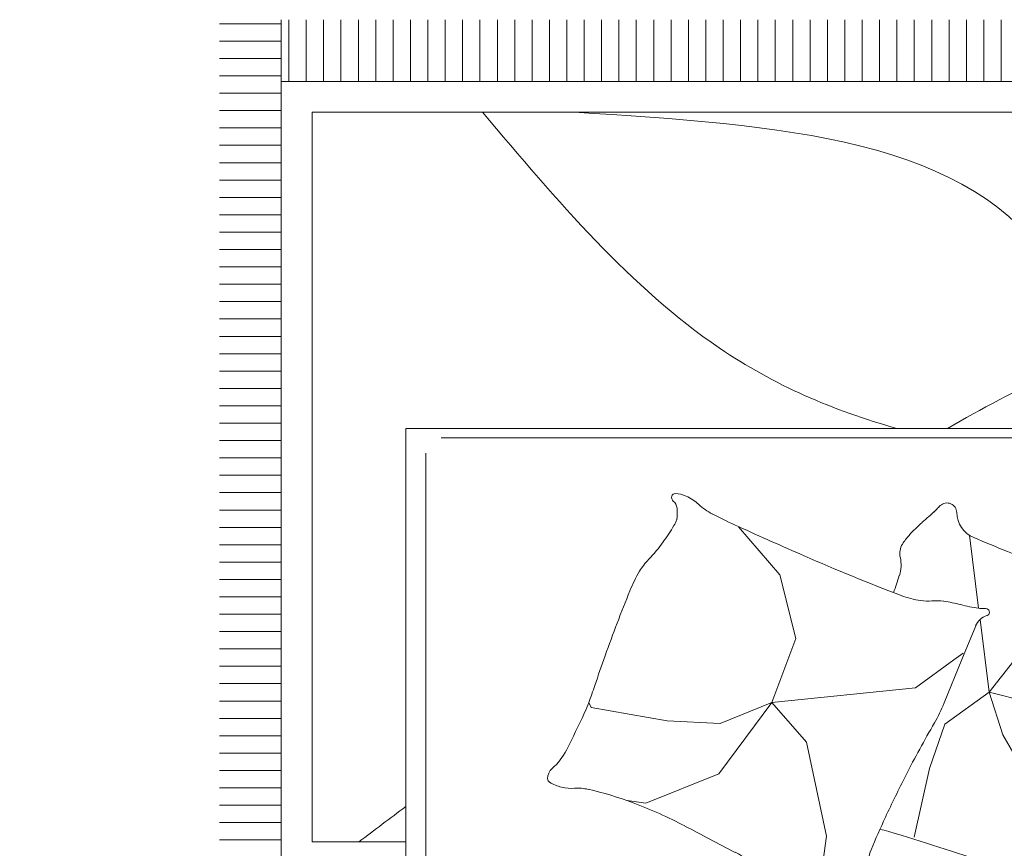
# Model space of a CAD drawing. Units: inches. Extents: x -7 to 1228, y -146 to 1091.
# Tile 38 of 88: x 1006 to 1045, y 117 to 150. Entities that reach past the tile are written whole.
import ezdxf

# ---------------------------------------------------------------- set-up
doc = ezdxf.new("R2010")
doc.units = ezdxf.units.IN
doc.layers.add('A-FURN', color=8, linetype='Continuous', lineweight=18)
doc.styles.add('DIM_FONT', font='SIMPLEX.shx', dxfattribs={"width": 0.8})

# ---------------------------------------------------------------- blocks, each defined once
blk = doc.blocks.new('A$C4F634EDD')
for p, q in [((0, 2.6295), (0, 2.2295)), ((0.5, 2.6295), (0, 2.6295)), ((0.5, 2.6295), (2.3, 2.6295)), ((0.5, 0.5295), (0.5, 2.6295)), ((0.5, 2.2295), (0.5, 2.6295)), ((2.3, 2.6295), (2.3, 0.5295)), ((2.3, 2.6295), (2.8, 2.6295)), ((2.3, 2.2295), (2.3, 2.6295)), ((2.8, 2.6295), (2.8, 2.2295)), ((0.5, 2.5771), (2.3, 2.5771)), ((2.392, 2.5115), (2.5692, 2.5765)), ((2.5692, 2.5765), (2.574, 2.5743)), ((0.2457, 2.5697), (0.2457, 2.4733)), ((2.4985, 2.5445), (2.5516, 2.564)), ((2.5516, 2.564), (2.5637, 2.5584)), ((2.574, 2.5743), (2.6638, 2.3298)), ((2.5062, 2.5454), (2.5487, 2.561)), ((2.5483, 2.5347), (2.5487, 2.561)), ((2.5487, 2.561), (2.5571, 2.56)), ((2.5615, 2.5536), (2.5514, 2.5318)), ((2.5571, 2.56), (2.5615, 2.5536)), ((2.5615, 2.5536), (2.5791, 2.5058)), ((2.5637, 2.5584), (2.6418, 2.3458)), ((2.4946, 2.5331), (2.4985, 2.5445)), ((2.5062, 2.5454), (2.5004, 2.5392)), ((2.5004, 2.5392), (2.5013, 2.5315)), ((2.5235, 2.5256), (2.5062, 2.5454)), ((2.5734, 2.3187), (2.4946, 2.5331)), ((2.5013, 2.5315), (2.5188, 2.4836)), ((2.5013, 2.5315), (2.5231, 2.5214)), ((2.5231, 2.5214), (2.5235, 2.5256)), ((2.5483, 2.5347), (2.5235, 2.5256)), ((2.5514, 2.5318), (2.5483, 2.5347)), ((2.5807, 2.4521), (2.5514, 2.5318)), ((2.412, 2.5007), (2.4634, 2.5196)), ((2.4634, 2.5196), (2.4875, 2.454)), ((2.4842, 2.5232), (2.47, 2.518)), ((2.47, 2.518), (2.472, 2.5127)), ((2.472, 2.5127), (2.4862, 2.5179)), ((2.4881, 2.5126), (2.4739, 2.5074)), ((2.4862, 2.5179), (2.4842, 2.5232)), ((2.4901, 2.5073), (2.4881, 2.5126)), ((2.5523, 2.4417), (2.5231, 2.5214)), ((2.3898, 2.5066), (2.392, 2.5115)), ((2.4795, 2.2621), (2.3898, 2.5066)), ((2.4361, 2.4352), (2.412, 2.5007)), ((2.4739, 2.5074), (2.4759, 2.502)), ((2.4759, 2.502), (2.4901, 2.5073)), ((2.492, 2.5019), (2.4778, 2.4967)), ((2.494, 2.4966), (2.492, 2.5019)), ((2.5791, 2.5058), (2.5788, 2.4956)), ((2.4778, 2.4967), (2.4798, 2.4914)), ((2.4798, 2.4914), (2.494, 2.4966)), ((2.4959, 2.4913), (2.4817, 2.4861)), ((2.4979, 2.486), (2.4959, 2.4913)), ((2.5788, 2.4956), (2.5767, 2.4848)), ((2.4817, 2.4861), (2.4837, 2.4808)), ((2.4837, 2.4808), (2.4979, 2.486)), ((2.4998, 2.4807), (2.4856, 2.4755)), ((2.4856, 2.4755), (2.4876, 2.4702)), ((2.4876, 2.4702), (2.5018, 2.4754)), ((2.5018, 2.4754), (2.4998, 2.4807)), ((2.5188, 2.4836), (2.5256, 2.4761)), ((2.5256, 2.4761), (2.5342, 2.4692)), ((2.5767, 2.4848), (2.5795, 2.4717)), ((2.5037, 2.47), (2.4895, 2.4648)), ((2.4895, 2.4648), (2.4915, 2.4595)), ((2.4915, 2.4595), (2.5057, 2.4647)), ((2.5057, 2.4647), (2.5037, 2.47)), ((2.5342, 2.4692), (2.5405, 2.4574)), ((2.5795, 2.4717), (2.586, 2.454)), ((2.4875, 2.454), (2.4361, 2.4352)), ((2.5405, 2.4574), (2.547, 2.4397)), ((2.5807, 2.4521), (2.6158, 2.3564)), ((2.5984, 2.4204), (2.586, 2.454)), ((2.5594, 2.4061), (2.547, 2.4397)), ((2.5523, 2.4417), (2.5875, 2.346)), ((2.4634, 2.4211), (2.474, 2.425)), ((2.474, 2.425), (2.4779, 2.4143)), ((2.4811, 2.4276), (2.4917, 2.4315)), ((2.485, 2.4169), (2.4811, 2.4276)), ((2.4917, 2.4315), (2.4956, 2.4208)), ((0.0957, 2.4197), (0.192, 2.4197)), ((0.2994, 2.4197), (0.3957, 2.4197)), ((2.4457, 2.4146), (2.4563, 2.4185)), ((2.4496, 2.4039), (2.4457, 2.4146)), ((2.4563, 2.4185), (2.4602, 2.4078)), ((2.4673, 2.4104), (2.4634, 2.4211)), ((2.4779, 2.4143), (2.4673, 2.4104)), ((2.4956, 2.4208), (2.485, 2.4169)), ((2.4883, 2.4081), (2.4989, 2.412)), ((2.4989, 2.412), (2.5028, 2.4014)), ((2.6047, 2.4086), (2.5984, 2.4204)), ((2.4602, 2.4078), (2.4496, 2.4039)), ((2.4528, 2.3951), (2.4635, 2.399)), ((2.4635, 2.399), (2.4674, 2.3883)), ((2.4706, 2.4016), (2.4812, 2.4055)), ((2.4745, 2.3909), (2.4706, 2.4016)), ((2.4812, 2.4055), (2.4851, 2.3949)), ((2.4922, 2.3975), (2.4883, 2.4081)), ((2.5028, 2.4014), (2.4922, 2.3975)), ((2.5622, 2.393), (2.5594, 2.4061)), ((2.6133, 2.4017), (2.6047, 2.4086)), ((2.6201, 2.3941), (2.6133, 2.4017)), ((2.6499, 2.3979), (2.6397, 2.3953)), ((2.6551, 2.397), (2.6499, 2.3979)), ((2.4567, 2.3844), (2.4528, 2.3951)), ((2.4674, 2.3883), (2.4567, 2.3844)), ((2.4851, 2.3949), (2.4745, 2.3909)), ((2.4777, 2.3821), (2.4883, 2.386)), ((2.4883, 2.386), (2.4922, 2.3754)), ((2.4954, 2.3886), (2.5061, 2.3925)), ((2.4993, 2.378), (2.4954, 2.3886)), ((2.5061, 2.3925), (2.51, 2.3819)), ((2.5601, 2.3822), (2.5622, 2.393)), ((2.6376, 2.3463), (2.6201, 2.3941)), ((2.6417, 2.39), (2.6488, 2.391)), ((2.6488, 2.391), (2.6538, 2.3895)), ((2.6538, 2.3895), (2.6596, 2.388)), ((2.6627, 2.392), (2.6551, 2.397)), ((2.6596, 2.388), (2.6626, 2.3867)), ((2.6626, 2.3867), (2.6662, 2.388)), ((2.6692, 2.394), (2.6627, 2.392)), ((2.6662, 2.388), (2.6632, 2.3828)), ((2.6736, 2.3944), (2.6692, 2.394)), ((2.6765, 2.391), (2.6736, 2.3944)), ((2.6742, 2.3795), (2.6765, 2.391)), ((2.6824, 2.3858), (2.6742, 2.3795)), ((2.6873, 2.3815), (2.6824, 2.3858)), ((2.46, 2.3756), (2.4706, 2.3795)), ((2.4639, 2.365), (2.46, 2.3756)), ((2.4706, 2.3795), (2.4745, 2.3689)), ((2.4816, 2.3715), (2.4777, 2.3821)), ((2.4922, 2.3754), (2.4816, 2.3715)), ((2.51, 2.3819), (2.4993, 2.378)), ((2.5026, 2.3691), (2.5132, 2.373)), ((2.5132, 2.373), (2.5171, 2.3624)), ((2.5238, 2.3769), (2.538, 2.3821)), ((2.5277, 2.3663), (2.5238, 2.3769)), ((2.538, 2.3821), (2.5419, 2.3715)), ((2.5598, 2.372), (2.5601, 2.3822)), ((2.5774, 2.3242), (2.5598, 2.372)), ((2.6632, 2.3828), (2.6736, 2.3744)), ((2.6736, 2.3744), (2.6922, 2.3593)), ((2.6853, 2.369), (2.6873, 2.3815)), ((2.6946, 2.376), (2.6853, 2.369)), ((2.6995, 2.3713), (2.6946, 2.376)), ((0.2457, 2.366), (0.2457, 2.2697)), ((2.4745, 2.3689), (2.4639, 2.365)), ((2.4672, 2.3561), (2.4778, 2.36)), ((2.4778, 2.36), (2.4817, 2.3494)), ((2.4849, 2.3626), (2.4955, 2.3665)), ((2.4888, 2.352), (2.4849, 2.3626)), ((2.4955, 2.3665), (2.4994, 2.3559)), ((2.5065, 2.3585), (2.5026, 2.3691)), ((2.5171, 2.3624), (2.5065, 2.3585)), ((2.5419, 2.3715), (2.5277, 2.3663)), ((2.6922, 2.3593), (2.7051, 2.3473)), ((2.695, 2.3603), (2.6995, 2.3713)), ((2.7031, 2.3682), (2.695, 2.3603)), ((2.7096, 2.3616), (2.7031, 2.3682)), ((2.7062, 2.351), (2.7096, 2.3616)), ((2.4711, 2.3455), (2.4672, 2.3561)), ((2.4817, 2.3494), (2.4711, 2.3455)), ((2.4994, 2.3559), (2.4888, 2.352)), ((2.6154, 2.3522), (2.5905, 2.3431)), ((2.6158, 2.3564), (2.6154, 2.3522)), ((2.6154, 2.3522), (2.6327, 2.3324)), ((2.6376, 2.3463), (2.6158, 2.3564)), ((2.6385, 2.3386), (2.6376, 2.3463)), ((2.7051, 2.3473), (2.7079, 2.3475)), ((2.7147, 2.3578), (2.7062, 2.351)), ((2.7079, 2.3475), (2.7079, 2.3443)), ((2.7214, 2.3517), (2.7147, 2.3578)), ((2.7196, 2.34), (2.7214, 2.3517)), ((2.7286, 2.3466), (2.7196, 2.34)), ((2.7346, 2.3423), (2.7286, 2.3466)), ((2.5774, 2.3242), (2.5875, 2.346)), ((2.5875, 2.346), (2.5905, 2.3431)), ((2.5905, 2.3431), (2.5901, 2.3168)), ((2.6327, 2.3324), (2.6385, 2.3386)), ((2.6418, 2.3458), (2.6369, 2.332)), ((2.7079, 2.3443), (2.727, 2.3277)), ((2.732, 2.3295), (2.7346, 2.3423)), ((2.7423, 2.3345), (2.732, 2.3295)), ((2.7495, 2.325), (2.7423, 2.3345)), ((0, 2.3301), (0.5, 2.3301)), ((2.8, 2.3301), (2.3, 2.3301)), ((2.5818, 2.3178), (2.5774, 2.3242)), ((2.6104, 2.3222), (2.5855, 2.3131)), ((2.5901, 2.3168), (2.6097, 2.324)), ((2.613, 2.3312), (2.6077, 2.3293)), ((2.6077, 2.3293), (2.6135, 2.3141)), ((2.6192, 2.3174), (2.613, 2.3312)), ((2.6153, 2.3261), (2.6327, 2.3324)), ((2.6369, 2.332), (2.6161, 2.3243)), ((2.6616, 2.3249), (2.6234, 2.3109)), ((2.6638, 2.3298), (2.6616, 2.3249)), ((2.727, 2.3277), (2.7512, 2.2983)), ((2.7406, 2.3172), (2.7495, 2.325)), ((2.7519, 2.3218), (2.7406, 2.3172)), ((2.7575, 2.3144), (2.7519, 2.3218)), ((2.6172, 2.3086), (2.4844, 2.2599)), ((2.561, 2.3141), (2.5433, 2.3076)), ((2.5649, 2.3035), (2.561, 2.3141)), ((2.5855, 2.3131), (2.5734, 2.3187)), ((2.5901, 2.3168), (2.5818, 2.3178)), ((2.6135, 2.3141), (2.6244, 2.2977)), ((2.626, 2.3069), (2.6192, 2.3174)), ((2.7526, 2.3045), (2.7575, 2.3144)), ((2.7622, 2.308), (2.7526, 2.3045)), ((2.7673, 2.2997), (2.7622, 2.308)), ((2.5114, 2.2959), (2.4936, 2.2894)), ((2.5153, 2.2853), (2.5114, 2.2959)), ((2.5362, 2.305), (2.5185, 2.2985)), ((2.5185, 2.2985), (2.5224, 2.2879)), ((2.5401, 2.2944), (2.5362, 2.305)), ((2.5433, 2.3076), (2.5472, 2.297)), ((2.5472, 2.297), (2.5649, 2.3035)), ((2.6244, 2.2977), (2.6349, 2.2825)), ((2.6365, 2.2916), (2.626, 2.3069)), ((2.7512, 2.2983), (2.756, 2.2695)), ((2.7574, 2.2924), (2.7673, 2.2997)), ((2.4936, 2.2894), (2.4976, 2.2788)), ((2.4976, 2.2788), (2.5153, 2.2853)), ((2.5224, 2.2879), (2.5401, 2.2944)), ((2.6407, 2.2834), (2.6365, 2.2916)), ((2.6438, 2.2739), (2.6407, 2.2834)), ((2.7687, 2.2905), (2.7574, 2.2924)), ((2.7587, 2.279), (2.7699, 2.2828)), ((2.7699, 2.2828), (2.7687, 2.2905)), ((0.5953, 2.1912), (0.616, 2.2738)), ((1.4546, 2.1912), (1.4752, 2.2738)), ((2.6349, 2.2825), (2.638, 2.273)), ((2.6399, 2.2712), (2.6374, 2.2659)), ((2.638, 2.273), (2.6399, 2.2712)), ((2.6519, 2.2716), (2.6438, 2.2739)), ((2.6535, 2.2628), (2.6519, 2.2716)), ((2.7708, 2.2725), (2.7587, 2.279)), ((2.7706, 2.2643), (2.7708, 2.2725)), ((2.4844, 2.2599), (2.4795, 2.2621)), ((2.6374, 2.2659), (2.6398, 2.257)), ((2.6398, 2.257), (2.6509, 2.259)), ((2.6509, 2.259), (2.6431, 2.2492)), ((2.6636, 2.2409), (2.6535, 2.2628)), ((2.756, 2.2695), (2.7459, 2.2483)), ((2.759, 2.2637), (2.7706, 2.2643)), ((2.7676, 2.2559), (2.759, 2.2637)), ((2.6431, 2.2492), (2.6473, 2.2398)), ((2.7459, 2.2483), (2.7284, 2.2317)), ((2.7529, 2.2505), (2.7645, 2.2498)), ((2.7607, 2.2424), (2.7529, 2.2505)), ((2.7645, 2.2498), (2.7676, 2.2559)), ((2.6473, 2.2398), (2.6592, 2.2429)), ((2.6592, 2.2429), (2.6521, 2.2314)), ((2.6836, 2.2287), (2.6636, 2.2409)), ((2.7284, 2.2317), (2.7063, 2.2256)), ((2.7509, 2.2314), (2.7459, 2.2418)), ((2.7459, 2.2418), (2.7568, 2.2352)), ((2.7568, 2.2352), (2.7607, 2.2424)), ((0, 2.2295), (0.5, 2.2295)), ((2.8, 2.2295), (2.3, 2.2295)), ((2.6521, 2.2314), (2.6598, 2.2248)), ((2.6598, 2.2248), (2.6697, 2.2309)), ((2.6697, 2.2309), (2.6684, 2.219)), ((2.6684, 2.219), (2.6761, 2.2145)), ((2.6761, 2.2145), (2.6821, 2.2237)), ((2.6821, 2.2237), (2.6843, 2.2135)), ((2.7063, 2.2256), (2.6836, 2.2287)), ((2.6927, 2.2117), (2.6986, 2.222)), ((2.6986, 2.222), (2.7019, 2.2098)), ((2.7102, 2.2104), (2.7113, 2.2218)), ((2.7113, 2.2218), (2.7192, 2.2137)), ((2.7255, 2.2152), (2.7242, 2.2265)), ((2.7242, 2.2265), (2.7324, 2.2165)), ((2.7324, 2.2165), (2.7386, 2.2208)), ((2.7386, 2.2208), (2.7354, 2.2306)), ((2.7354, 2.2306), (2.7462, 2.2264)), ((2.7462, 2.2264), (2.7509, 2.2314)), ((2.6843, 2.2135), (2.6927, 2.2117)), ((2.7019, 2.2098), (2.7102, 2.2104)), ((2.7192, 2.2137), (2.7255, 2.2152)), ((0.5878, 2.1612), (0.5953, 2.1912)), ((1.4471, 2.1612), (1.4546, 2.1912)), ((1.5035, 2.141), (0.5458, 2.141)), ((1.5035, 2.141), (2.2716, 1.7136)), ((0.5258, 2.121), (0.5258, 0.5617)), ((1.576, 1.9433), (1.5624, 1.8479)), ((0.5458, 1.8684), (1.5653, 1.8684)), ((1.5624, 1.8479), (1.5641, 1.7178)), ((2.2716, 0.5617), (2.2716, 1.7136)), ((0.2586, 1.1753), (0.3386, 1.1753)), ((0.3386, 0), (0.3386, 1.1852)), ((0.3486, 1.1052), (0.3486, 1.1852)), ((0.3711, 1.1052), (0.3711, 1.1852)), ((0.3936, 1.1052), (0.3936, 1.1852)), ((0.4161, 1.1052), (0.4161, 1.1852)), ((0.4386, 1.1052), (0.4386, 1.1852)), ((0.4611, 1.1052), (0.4611, 1.1852)), ((0.4836, 1.1052), (0.4836, 1.1852)), ((2.3061, 1.1052), (2.3061, 1.1852)), ((2.3286, 1.1052), (2.3286, 1.1852)), ((2.3511, 1.1052), (2.3511, 1.1852)), ((2.3736, 1.1052), (2.3736, 1.1852)), ((2.3961, 1.1052), (2.3961, 1.1852)), ((2.4186, 1.1052), (2.4186, 1.1852)), ((2.4411, 1.1052), (2.4411, 1.1852)), ((2.4588, 1.1852), (2.4588, 0)), ((2.4588, 1.1753), (2.5388, 1.1753)), ((1.031, 1.1612), (1.0448, 1.0581)), ((1.4276, 1.1611), (1.3484, 1.0571)), ((0.2586, 1.1528), (0.3386, 1.1528)), ((2.4588, 1.1528), (2.5388, 1.1528)), ((0.2586, 1.1303), (0.3386, 1.1303)), ((2.4588, 1.1303), (2.5388, 1.1303)), ((0.2586, 1.1078), (0.3386, 1.1078)), ((0.3386, 1.1052), (0.5, 1.1052)), ((2.3, 1.1052), (2.4588, 1.1052)), ((2.4588, 1.1078), (2.5388, 1.1078)), ((0.2586, 1.0853), (0.3386, 1.0853)), ((2.4588, 1.0853), (2.5388, 1.0853)), ((0.2586, 1.0628), (0.3386, 1.0628)), ((0.3786, 1.0652), (0.5, 1.0652)), ((0.3786, 0.12), (0.3786, 1.0652)), ((1.1784, 0.9702), (1.1586, 1.0591)), ((2.3, 1.0652), (2.4188, 1.0652)), ((2.4188, 1.0652), (2.4188, 0.12)), ((2.4588, 1.0628), (2.5388, 1.0628)), ((1.0448, 1.0581), (1.019, 0.936)), ((1.3484, 1.0571), (1.2733, 0.9268)), ((0.2586, 1.0403), (0.3386, 1.0403)), ((2.4588, 1.0403), (2.5388, 1.0403)), ((0.2586, 1.0178), (0.3386, 1.0178)), ((0.8108, 1.0151), (0.7868, 1.0117)), ((0.9054, 0.9773), (0.8108, 1.0151)), ((2.4588, 1.0178), (2.5388, 1.0178)), ((0.2586, 0.9953), (0.3386, 0.9953)), ((2.4588, 0.9953), (2.5388, 0.9953)), ((0.2586, 0.9728), (0.3386, 0.9728)), ((0.9743, 0.8845), (0.9054, 0.9773)), ((1.1982, 0.9129), (1.1784, 0.9702)), ((2.4588, 0.9728), (2.5388, 0.9728)), ((0.2586, 0.9503), (0.3386, 0.9503)), ((2.4588, 0.9503), (2.5388, 0.9503)), ((1.019, 0.936), (0.9743, 0.8845)), ((0.2586, 0.9278), (0.3386, 0.9278)), ((1.2733, 0.9268), (1.2555, 0.8715)), ((2.4588, 0.9278), (2.5388, 0.9278)), ((0.8384, 0.9085), (0.7403, 0.8913)), ((0.9072, 0.912), (0.8384, 0.9085)), ((0.9743, 0.8845), (0.9072, 0.912)), ((1.2555, 0.8715), (1.1982, 0.9129)), ((0.2586, 0.9053), (0.3386, 0.9053)), ((1.2555, 0.8715), (1.384, 0.9031)), ((1.384, 0.9031), (1.4868, 0.8892)), ((2.4588, 0.9053), (2.5388, 0.9053)), ((0.2586, 0.8828), (0.3386, 0.8828)), ((0.7403, 0.8913), (0.737, 0.8849)), ((0.9743, 0.8845), (1.0052, 0.802)), ((0.9743, 0.8845), (1.16, 0.8656)), ((1.1973, 0.8853), (1.2203, 0.829)), ((1.4868, 0.8892), (1.5228, 0.8692)), ((2.4588, 0.8828), (2.5388, 0.8828)), ((1.2555, 0.8715), (1.2437, 0.7773)), ((1.2555, 0.8715), (1.3049, 0.8082)), ((0.2586, 0.8603), (0.3386, 0.8603)), ((1.16, 0.8656), (1.2099, 0.8295)), ((2.4588, 0.8603), (2.5388, 0.8603)), ((0.2586, 0.8378), (0.3386, 0.8378)), ((1.2099, 0.8295), (1.222, 0.8209)), ((1.2203, 0.829), (1.2381, 0.7855)), ((2.4588, 0.8378), (2.5388, 0.8378)), ((0.2586, 0.8153), (0.3386, 0.8153)), ((1.3049, 0.8082), (1.3701, 0.7608)), ((2.4588, 0.8153), (2.5388, 0.8153)), ((0.2586, 0.7928), (0.3386, 0.7928)), ((1.0052, 0.802), (0.9846, 0.7194)), ((2.4588, 0.7928), (2.5388, 0.7928)), ((0.2586, 0.7703), (0.3386, 0.7703)), ((2.4588, 0.7703), (2.5388, 0.7703)), ((1.2419, 0.7626), (1.23, 0.668)), ((1.3701, 0.7608), (1.463, 0.7608)), ((0.2586, 0.7478), (0.3386, 0.7478)), ((2.4588, 0.7478), (2.5388, 0.7478)), ((0.2586, 0.7253), (0.3386, 0.7253)), ((0.9846, 0.7194), (0.931, 0.6569)), ((2.4588, 0.7253), (2.5388, 0.7253)), ((0.2586, 0.7028), (0.3386, 0.7028)), ((2.4588, 0.7028), (2.5388, 0.7028)), ((0.2586, 0.6803), (0.3386, 0.6803)), ((2.4588, 0.6803), (2.5388, 0.6803)), ((0.2586, 0.6578), (0.3386, 0.6578)), ((2.4588, 0.6578), (2.5388, 0.6578)), ((0.2586, 0.6353), (0.3386, 0.6353)), ((2.4588, 0.6353), (2.5388, 0.6353)), ((0.2586, 0.6128), (0.3386, 0.6128)), ((2.4588, 0.6128), (2.5388, 0.6128)), ((0.2586, 0.5903), (0.3386, 0.5903)), ((2.4588, 0.5903), (2.5388, 0.5903)), ((0.2586, 0.5678), (0.3386, 0.5678)), ((2.4588, 0.5678), (2.5388, 0.5678)), ((0.2586, 0.5453), (0.3386, 0.5453)), ((0.5458, 0.5417), (2.2516, 0.5417)), ((2.4588, 0.5453), (2.5388, 0.5453)), ((2.3, 0.5295), (0.5, 0.5295)), ((0.2586, 0.5228), (0.3386, 0.5228)), ((2.4588, 0.5228), (2.5388, 0.5228)), ((0.2586, 0.5003), (0.3386, 0.5003)), ((2.4588, 0.5003), (2.5388, 0.5003)), ((0.2586, 0.4778), (0.3386, 0.4778)), ((2.4588, 0.4778), (2.5388, 0.4778)), ((0.2586, 0.4553), (0.3386, 0.4553)), ((2.4588, 0.4553), (2.5388, 0.4553)), ((0.2586, 0.4328), (0.3386, 0.4328)), ((2.4588, 0.4328), (2.5388, 0.4328)), ((0.2586, 0.4103), (0.3386, 0.4103)), ((2.4588, 0.4103), (2.5388, 0.4103)), ((0.2586, 0.3878), (0.3386, 0.3878)), ((2.4588, 0.3878), (2.5388, 0.3878)), ((0.2586, 0.3653), (0.3386, 0.3653)), ((2.4588, 0.3653), (2.5388, 0.3653)), ((0.2586, 0.3428), (0.3386, 0.3428)), ((2.4588, 0.3428), (2.5388, 0.3428)), ((0.2586, 0.3203), (0.3386, 0.3203)), ((2.4588, 0.3203), (2.5388, 0.3203)), ((0.2586, 0.2978), (0.3386, 0.2978)), ((2.4588, 0.2978), (2.5388, 0.2978)), ((0.2586, 0.2753), (0.3386, 0.2753)), ((2.4588, 0.2753), (2.5388, 0.2753)), ((0.2586, 0.2528), (0.3386, 0.2528)), ((2.4588, 0.2528), (2.5388, 0.2528)), ((0.2586, 0.2303), (0.3386, 0.2303)), ((2.4588, 0.2303), (2.5388, 0.2303)), ((0.2586, 0.2078), (0.3386, 0.2078)), ((2.4588, 0.2078), (2.5388, 0.2078)), ((0.2586, 0.1853), (0.3386, 0.1853)), ((2.4588, 0.1853), (2.5388, 0.1853)), ((0.2586, 0.1628), (0.3386, 0.1628)), ((2.4588, 0.1628), (2.5388, 0.1628)), ((0.2586, 0.1403), (0.3386, 0.1403)), ((2.4588, 0.1403), (2.5388, 0.1403)), ((0.2586, 0.1178), (0.3386, 0.1178)), ((2.4188, 0.12), (0.3786, 0.12)), ((2.4588, 0.1178), (2.5388, 0.1178)), ((0.2586, 0.0953), (0.3386, 0.0953)), ((2.4588, 0.0953), (2.5388, 0.0953)), ((2.4588, 0.08), (0.3386, 0.08)), ((0.3486, 0), (0.3486, 0.08)), ((0.3711, 0), (0.3711, 0.08)), ((0.3936, 0), (0.3936, 0.08)), ((0.4161, 0), (0.4161, 0.08)), ((0.4386, 0), (0.4386, 0.08)), ((0.4611, 0), (0.4611, 0.08)), ((0.4836, 0), (0.4836, 0.08)), ((0.5061, 0), (0.5061, 0.08)), ((0.5286, 0), (0.5286, 0.08)), ((0.5511, 0), (0.5511, 0.08)), ((0.5736, 0), (0.5736, 0.08)), ((0.5961, 0), (0.5961, 0.08)), ((0.6186, 0), (0.6186, 0.08)), ((0.6411, 0), (0.6411, 0.08)), ((0.6636, 0), (0.6636, 0.08)), ((0.6861, 0), (0.6861, 0.08)), ((0.7086, 0), (0.7086, 0.08)), ((0.7311, 0), (0.7311, 0.08)), ((0.7536, 0), (0.7536, 0.08)), ((0.7761, 0), (0.7761, 0.08)), ((0.7986, 0), (0.7986, 0.08)), ((0.8211, 0), (0.8211, 0.08)), ((0.8436, 0), (0.8436, 0.08)), ((0.8661, 0), (0.8661, 0.08)), ((0.8886, 0), (0.8886, 0.08)), ((0.9111, 0), (0.9111, 0.08)), ((0.9336, 0), (0.9336, 0.08)), ((0.9561, 0), (0.9561, 0.08)), ((0.9786, 0), (0.9786, 0.08)), ((1.0011, 0), (1.0011, 0.08)), ((1.0236, 0), (1.0236, 0.08)), ((1.0461, 0), (1.0461, 0.08)), ((1.0686, 0), (1.0686, 0.08)), ((1.0911, 0), (1.0911, 0.08)), ((1.1136, 0), (1.1136, 0.08)), ((1.1361, 0), (1.1361, 0.08)), ((1.1586, 0), (1.1586, 0.08)), ((1.1811, 0), (1.1811, 0.08)), ((1.2036, 0), (1.2036, 0.08)), ((1.2261, 0), (1.2261, 0.08)), ((1.2486, 0), (1.2486, 0.08)), ((1.2711, 0), (1.2711, 0.08)), ((1.2936, 0), (1.2936, 0.08)), ((1.3161, 0), (1.3161, 0.08)), ((1.3386, 0), (1.3386, 0.08)), ((1.3611, 0), (1.3611, 0.08)), ((1.3836, 0), (1.3836, 0.08)), ((1.4061, 0), (1.4061, 0.08)), ((1.4286, 0), (1.4286, 0.08)), ((1.4511, 0), (1.4511, 0.08)), ((1.4736, 0), (1.4736, 0.08)), ((1.4961, 0), (1.4961, 0.08)), ((1.5186, 0), (1.5186, 0.08)), ((1.5411, 0), (1.5411, 0.08)), ((1.5636, 0), (1.5636, 0.08)), ((1.5861, 0), (1.5861, 0.08)), ((1.6086, 0), (1.6086, 0.08)), ((1.6311, 0), (1.6311, 0.08)), ((1.6536, 0), (1.6536, 0.08)), ((1.6761, 0), (1.6761, 0.08)), ((1.6986, 0), (1.6986, 0.08)), ((1.7211, 0), (1.7211, 0.08)), ((1.7436, 0), (1.7436, 0.08)), ((1.7661, 0), (1.7661, 0.08)), ((1.7886, 0), (1.7886, 0.08)), ((1.8111, 0), (1.8111, 0.08)), ((1.8336, 0), (1.8336, 0.08)), ((1.8561, 0), (1.8561, 0.08)), ((1.8786, 0), (1.8786, 0.08)), ((1.9011, 0), (1.9011, 0.08)), ((1.9236, 0), (1.9236, 0.08)), ((1.9461, 0), (1.9461, 0.08)), ((1.9686, 0), (1.9686, 0.08)), ((1.9911, 0), (1.9911, 0.08)), ((2.0136, 0), (2.0136, 0.08)), ((2.0361, 0), (2.0361, 0.08)), ((2.0586, 0), (2.0586, 0.08)), ((2.0811, 0), (2.0811, 0.08)), ((2.1036, 0), (2.1036, 0.08)), ((2.1261, 0), (2.1261, 0.08)), ((2.1486, 0), (2.1486, 0.08)), ((2.1711, 0), (2.1711, 0.08)), ((2.1936, 0), (2.1936, 0.08)), ((2.2161, 0), (2.2161, 0.08)), ((2.2386, 0), (2.2386, 0.08)), ((2.2611, 0), (2.2611, 0.08)), ((2.2836, 0), (2.2836, 0.08)), ((2.3061, 0), (2.3061, 0.08)), ((2.3286, 0), (2.3286, 0.08)), ((2.3511, 0), (2.3511, 0.08)), ((2.3736, 0), (2.3736, 0.08)), ((2.3961, 0), (2.3961, 0.08)), ((2.4186, 0), (2.4186, 0.08)), ((2.4411, 0), (2.4411, 0.08)), ((0.2586, 0.0728), (0.3386, 0.0728)), ((2.4588, 0.0728), (2.5388, 0.0728)), ((0.2586, 0.0503), (0.3386, 0.0503)), ((2.4588, 0.0503), (2.5388, 0.0503)), ((0.2586, 0.0278), (0.3386, 0.0278)), ((2.4588, 0.0278), (2.5388, 0.0278)), ((0.2586, 0.0053), (0.3386, 0.0053)), ((2.4588, 0.0053), (2.5388, 0.0053))]:
    blk.add_line(p, q)
for radius in [0.1222, 0.0865]:
    blk.add_circle((0.2457, 2.4197), radius)
for centre, radius, start, end in [((0.5848, 2.5274), 0.0131, 101.2724, 206.5805), ((0.5999, 2.4516), 0.0904, 90, 101.2724), ((0.5999, 2.3808), 0.1611, 81.5628, 90), ((0.5788, 2.2388), 0.3048, 74.256, 81.5628), ((1.3132, 2.5864), 0.0539, 275.2592, 300.6513), ((1.3554, 2.5152), 0.0289, 85.6975, 120.6513), ((1.3556, 2.519), 0.0251, 68.2117, 85.6975), ((1.3647, 2.5395), 0.00232, 258.1069, 19.564), ((1.3637, 2.5391), 0.00342, 19.564, 68.2117), ((1.444, 2.5274), 0.0131, 101.2724, 206.5805), ((1.4591, 2.4516), 0.0904, 90, 101.2724), ((1.4591, 2.3808), 0.1611, 81.5628, 90), ((1.438, 2.2388), 0.3048, 74.256, 81.5628), ((2.1724, 2.5864), 0.0539, 275.2592, 300.6513), ((2.2146, 2.5152), 0.0289, 85.6975, 120.6513), ((2.2149, 2.519), 0.0251, 68.2117, 85.6975), ((2.224, 2.5395), 0.00232, 258.1069, 19.564), ((2.2229, 2.5391), 0.00342, 19.564, 68.2117), ((0.7272, 2.7653), 0.2422, 254.256, 262.4531), ((0.7851, 3.2019), 0.6827, 262.4531, 270), ((0.7851, 3.5682), 1.049, 270, 276.0867), ((0.8402, 3.0514), 0.5293, 276.0867, 280.1899), ((1.1602, -8.1346), 10.6675, 90.30153, 91.21582), ((1.1169, 2.2433), 0.2897, 85.1982, 92.5386), ((1.2142, 3.4021), 0.8732, 265.1982, 269.4243), ((1.3082, 2.3102), 0.234, 110.8603, 117.2396), ((1.2204, 4.0232), 1.4943, 269.4243, 271.9079), ((1.2995, 2.4357), 0.0992, 105.9352, 126.0864), ((1.2429, 3.3501), 0.8208, 271.9079, 275.2592), ((1.2995, 2.4357), 0.0992, 85.7841, 105.9352), ((1.3739, 2.5288), 0.0156, 158.0096, 201.421), ((1.3634, 2.533), 0.00428, 78.1069, 158.0096), ((1.5865, 2.7653), 0.2422, 254.256, 262.4531), ((1.6443, 3.2019), 0.6827, 262.4531, 270), ((1.6443, 3.5682), 1.049, 270, 276.0867), ((1.4785, 15.4878), 12.9656, 271.22425, 272.05324), ((1.97, 2.3805), 0.1524, 92.5386, 100.1899), ((1.9761, 2.2433), 0.2897, 85.1982, 92.5386), ((2.0734, 3.4021), 0.8732, 265.1982, 269.4243), ((2.1674, 2.3102), 0.234, 110.8603, 117.2396), ((2.0797, 4.0232), 1.4943, 269.4243, 271.9079), ((2.1588, 2.4357), 0.0992, 105.9352, 126.0864), ((2.1021, 3.3501), 0.8208, 271.9079, 275.2592), ((2.1588, 2.4357), 0.0992, 85.7841, 105.9352), ((2.2331, 2.5288), 0.0156, 158.0096, 201.421), ((2.2226, 2.533), 0.00428, 78.1069, 158.0096), ((0.6036, 2.5368), 0.0342, 206.5805, 265.5998), ((1.2362, 2.45), 0.0768, 117.2396, 128.3886), ((1.2995, 2.4357), 0.0992, 126.0864, 143.8234), ((1.3288, 2.5111), 0.0328, 351.8665, 21.421), ((1.4628, 2.5368), 0.0342, 206.5805, 265.5998), ((2.0954, 2.45), 0.0768, 117.2396, 128.3886), ((2.1588, 2.4357), 0.0992, 126.0864, 143.8234), ((2.1881, 2.5111), 0.0328, 351.8665, 21.421), ((1.0898, 2.4496), 0.4918, 173.7676, 180), ((0.5368, 2.3783), 0.1399, 45.0976, 62.7964), ((1.4317, 2.2032), 0.3916, 128.3886, 133.8115), ((1.1177, 2.5413), 0.246, 347.8905, 351.8665), ((1.949, 2.4496), 0.4918, 173.7676, 180), ((2.291, 2.2032), 0.3916, 128.3886, 133.8115), ((1.977, 2.5413), 0.246, 347.8905, 351.8665), ((0.5462, 2.4142), 0.0899, 41.4429, 53.7359), ((1.2995, 2.4357), 0.0992, 143.8234, 161.5603), ((1.5522, 2.448), 0.1983, 167.8905, 172.3191), ((2.1588, 2.4357), 0.0992, 143.8234, 161.5603), ((2.4114, 2.448), 0.1983, 167.8905, 172.3191), ((0.5368, 2.3783), 0.1399, 27.3988, 45.0976), ((1.3165, 2.3233), 0.2252, 133.8115, 140.9651), ((2.2605, 2.3525), 0.9131, 172.3191, 176.6313), ((2.1757, 2.3233), 0.2252, 133.8115, 140.9651), ((3.1198, 2.3525), 0.9131, 172.3191, 176.6313), ((0.5741, 2.4389), 0.0526, 25.3551, 41.4429), ((0.4851, 2.3967), 0.1511, 21.8149, 25.3551), ((1.1799, 2.4341), 0.0493, 140.9651, 151.6832), ((2.0391, 2.4341), 0.0493, 140.9651, 151.6832), ((0.8019, 2.4496), 0.204, 180, 189.6844), ((0.4345, 2.3765), 0.2056, 18.7799, 21.8149), ((1.3127, 2.3625), 0.2002, 151.6832, 156.9972), ((1.6611, 2.4496), 0.204, 180, 189.6844), ((2.1719, 2.3625), 0.2002, 151.6832, 156.9972), ((0.576, 2.4246), 0.0562, 0, 18.7799), ((0.5368, 2.3783), 0.1399, 16.515, 27.3988), ((0.5406, 2.4246), 0.0915, 345.3149, 0), ((1.4703, 2.5637), 0.882, 189.6844, 192.1984), ((0.5368, 2.3783), 0.1399, 5.6311, 16.515), ((2.3295, 2.5637), 0.882, 189.6844, 192.1984), ((2.0266, 2.3663), 0.6787, 176.6313, 181.6331), ((2.8858, 2.3663), 0.6787, 176.6313, 181.6331), ((0.2982, 2.3103), 0.3171, 8.0051, 12.1984), ((1.1575, 2.3103), 0.3171, 8.0051, 12.1984), ((-0.0401, 2.2627), 0.6588, 2.6649, 8.0051), ((2.7128, 2.3859), 1.3652, 181.6331, 183.055), ((0.8191, 2.2627), 0.6588, 2.6649, 8.0051), ((3.5721, 2.3859), 1.3652, 181.6331, 183.055), ((14.9657, 3.0398), 13.6356, 183.05496, 183.50486), ((15.8249, 3.0398), 13.6356, 183.05496, 183.50486), ((0.5503, 2.2902), 0.0677, 345.9548, 2.6649), ((1.4096, 2.2902), 0.0677, 345.9548, 2.6649), ((1.1303, 1.9835), 0.2721, 85.9172, 93.5552), ((1.1455, 2.197), 0.058, 69.3257, 85.9172), ((0.9871, 1.7772), 0.5066, 65.6735, 69.3257), ((0.6058, 0.9338), 1.4323, 63.5015, 65.6735), ((0.473, 2.8815), 0.7387, 293.4844, 295.3111), ((1.1054, 1.9358), 0.3126, 57.865, 63.5015), ((1.6762, 2.2258), 0.3212, 183.5049, 189.9984), ((1.3322, 2.8815), 0.7387, 293.4844, 295.3111), ((2.5355, 2.2258), 0.3212, 183.5049, 189.9984), ((0.473, 2.8815), 0.7387, 289.428, 291.6577), ((0.473, 2.8815), 0.7387, 291.6577, 293.4844), ((0.8841, 1.5835), 0.7286, 54.1737, 57.865), ((1.3322, 2.8815), 0.7387, 289.428, 291.6577), ((1.3322, 2.8815), 0.7387, 291.6577, 293.4844), ((0.473, 2.8815), 0.7387, 287.1982, 289.428), ((1.3322, 2.8815), 0.7387, 287.1982, 289.428), ((0.5763, 2.3896), 0.2297, 279.4841, 287.3864), ((0.6807, 2.0561), 0.1197, 96.4341, 107.3864), ((0.6836, 2.0301), 0.1459, 78.4414, 96.4341), ((0.759, 2.3985), 0.2301, 258.4414, 272.7491), ((0.7026, 3.5718), 1.4048, 272.7491, 274.6176), ((0.9136, 0.9591), 1.2165, 92.6096, 94.6176), ((1.2501, -19.8405), 22.0183, 90.37908, 91.01965), ((1.2012, -3.5404), 5.7185, 89.7135, 90.9704), ((1.224, 1.0141), 1.164, 86.426, 89.7135), ((1.2875, 2.0302), 0.1459, 77.131, 86.426), ((1.3099, 2.1283), 0.0453, 62.7159, 77.131), ((1.3658, 2.2367), 0.0767, 242.7159, 253.7788), ((1.3409, 2.1667), 0.0193, 343.3022, 9.9984), ((1.4355, 2.3896), 0.2297, 279.4841, 287.3864), ((1.5399, 2.0561), 0.1197, 96.4341, 107.3864), ((1.5429, 2.0301), 0.1459, 78.4414, 96.4341), ((1.6182, 2.3985), 0.2301, 258.4414, 272.7491), ((1.5619, 3.5718), 1.4048, 272.7491, 274.6176), ((1.7729, 0.9591), 1.2165, 92.6096, 94.6176), ((2.1093, -19.8405), 22.0183, 90.37908, 91.01965), ((2.0605, -3.5404), 5.7185, 89.7135, 90.9704), ((2.0833, 1.0141), 1.164, 86.426, 89.7135), ((2.1467, 2.0302), 0.1459, 77.131, 86.426), ((2.1691, 2.1283), 0.0453, 62.7159, 77.131), ((2.2251, 2.2367), 0.0767, 242.7159, 253.7788), ((2.2001, 2.1667), 0.0193, 343.3022, 9.9984), ((0.5887, 2.1609), 0.000917, 165.9551, 274.0829), ((0.5695, 2.4301), 0.2708, 274.0829, 279.4841), ((1.3688, 2.247), 0.0875, 253.7788, 262.8796), ((1.3581, 2.1615), 0.00132, 262.8796, 343.3022), ((1.448, 2.1609), 0.000917, 165.9551, 274.0829), ((1.4288, 2.4301), 0.2708, 274.0829, 279.4841), ((2.2281, 2.247), 0.0875, 253.7788, 262.8796), ((2.2174, 2.1615), 0.00132, 262.8796, 343.3022), ((0.5458, 2.121), 0.02, 90, 180), ((1.2147, 1.9017), 0.3751, 20.1488, 39.6445), ((1.3977, 1.9688), 0.1801, 351.8644, 20.1488), ((0.5458, 1.8884), 0.02, 180, 270), ((1.4194, 4.2174), 2.5158, 281.6741, 283.1904), ((2.0378, 1.5789), 0.1942, 97.7304, 103.1904), ((2.0195, 1.7137), 0.0581, 79.2724, 97.7304), ((1.2737, -2.2227), 4.0646, 77.0745, 79.2724), ((0.6102, 18.0525), 16.3521, 273.75703, 274.62393), ((1.0582, 5.4638), 3.7801, 277.692, 279.495), ((2.0359, 1.0981), 0.6574, 74.0648, 77.0745), ((1.7125, -0.0344), 1.8351, 72.2636, 74.0648), ((1.0348, 1.1521), 0.0127, 51.1864, 183.2455), ((0.9991, 1.1077), 0.0697, 45.8726, 51.1864), ((1.4251, 1.1259), 0.0352, 86.0516, 110.3452), ((1.4273, 1.1567), 0.00443, 13.2808, 86.0516), ((0.9863, 1.1494), 0.0359, 297.2902, 3.2455), ((1.0791, 1.1902), 0.0452, 225.8726, 232.4713), ((1.2846, 1.4577), 0.3825, 232.4713, 233.7837), ((0.6683, 0.6162), 0.6605, 52.7849, 53.7837), ((1.3469, 1.2115), 0.0792, 292.7069, 308.5854), ((1.4338, 1.1026), 0.0601, 110.3452, 128.5854), ((1.4376, 1.1398), 0.0142, 126.5792, 169.5926), ((1.4254, 1.1562), 0.0063, 306.5792, 13.2808), ((0.9362, 0.9689), 0.2176, 46.4776, 52.7849), ((1.0543, 1.9106), 0.8371, 290.1287, 292.7069), ((1.4996, 1.1284), 0.0771, 169.5926, 177.2714), ((1.0327, 1.0706), 0.0774, 35.8936, 46.4776), ((-0.4107, 5.9078), 5.0942, 289.0836, 290.1287), ((1.4378, 1.1314), 0.0153, 177.2714, 194.5709), ((1.4611, 1.1374), 0.0393, 194.5709, 206.8179), ((-0.4173, 3.8699), 3.0972, 296.4147, 297.2902), ((1.0771, 1.1027), 0.0226, 351.9508, 35.8936), ((1.7401, 1.2785), 0.352, 206.8179, 210.9056), ((1.1449, 1.0931), 0.0458, 171.9508, 202.4162), ((1.6045, 1.1973), 0.194, 210.9056, 219.7005), ((1.8575, -0.7096), 2.0162, 116.4147, 117.4999), ((0.2266, 4.0657), 3.145, 286.6085, 289.0836), ((3.744, -4.3336), 6.1019, 117.49986, 117.84822), ((2.032, 1.4591), 1.0054, 202.4162, 205.0529), ((1.3929, 1.0217), 0.081, 26.0735, 39.7005), ((-1.8336, 6.2238), 5.8383, 297.49208, 297.84822), ((1.0922, 1.1636), 0.1166, 280.7366, 286.6085), ((1.2892, 0.9709), 0.1965, 17.8396, 26.0735), ((0.5736, 1.5979), 0.6236, 290.7486, 297.4921), ((2.6493, 1.7476), 1.6868, 205.0529, 207.0884), ((-0.4304, 0.4175), 2.003, 15.2625, 17.8396), ((0.6422, 1.4168), 0.43, 282.6252, 290.7486), ((0.7152, 0.9361), 0.0599, 86.6119, 103.0402), ((0.7224, 1.0587), 0.063, 266.6119, 282.6252), ((0.6894, 0.9832), 0.0058, 121.6917, 179.0386), ((0.7004, 0.983), 0.0168, 179.0386, 229.4914), ((0.7131, 0.9448), 0.0509, 103.0402, 121.6917), ((0.6405, 0.9128), 0.0755, 26.3332, 49.4914), ((2.541, 1.6922), 1.5652, 207.0884, 209.936), ((-1.6775, -0.2344), 2.6619, 25.1732, 26.3332), ((-0.0881, 0.5109), 1.6481, 13.841, 15.2625), ((0.9989, 0.8042), 0.2143, 22.2355, 29.936), ((0.5689, 0.8213), 0.1798, 20.7081, 25.1732), ((2.0418, 1.0357), 0.5454, 193.841, 196.3122), ((0.2268, 0.692), 0.5454, 18.2369, 20.7081), ((1.6908, 0.933), 0.1798, 196.3122, 200.7773), ((4.0115, 1.8135), 2.6619, 200.7773, 201.9373), ((2.3102, 1.3785), 1.6481, 198.2369, 199.6584), ((2.6444, 1.4979), 2.003, 199.6584, 202.2355), ((1.6124, 0.8472), 0.0755, 201.9373, 225.0955), ((1.5473, 0.7819), 0.0168, 354.6428, 45.0955), ((1.2594, 0.7942), 0.0231, 202.2355, 252.8133), ((1.5582, 0.7808), 0.0058, 297.2959, 354.6428), ((1.2512, 0.7678), 0.00467, 289.3799, 72.8133), ((1.5721, 0.3449), 0.43, 98.2293, 106.3527), ((1.5195, 0.708), 0.063, 82.216, 98.2293), ((1.5362, 0.8298), 0.0599, 262.216, 278.6443), ((1.5375, 0.8209), 0.0509, 278.6443, 297.2959), ((1.1834, 0.6373), 0.1166, 98.1216, 111.0043), ((1.1763, 0.687), 0.0663, 85.4882, 98.1216), ((1.1871, 0.8241), 0.0712, 265.4882, 277.6784), ((1.1727, 0.9313), 0.1794, 277.6784, 284.8807), ((1.2689, 0.569), 0.1955, 97.9822, 104.8807), ((1.2465, 0.729), 0.034, 85.7407, 97.9822), ((1.2497, 0.772), 0.0092, 265.7407, 289.3799), ((1.6266, 0.159), 0.6236, 106.3527, 113.0962), ((0.9722, 0.8143), 0.1965, 202.2355, 210.4694), ((2.2689, -2.1899), 3.145, 111.0043, 113.4795), ((0.1831, 0.4093), 1.0054, 18.0203, 19.3448), ((3.6722, -4.6377), 5.8383, 113.0962, 113.45234), ((0.8727, 0.7557), 0.081, 210.4694, 224.0964), ((1.0957, 0.7061), 0.0458, 347.5549, 18.0203), ((-1.0798, 6.3161), 6.1019, 293.10398, 293.45234), ((0.5234, 2.5582), 2.0162, 292.0188, 293.104), ((0.6752, 0.5644), 0.194, 35.3015, 44.0964), ((3.0455, -3.9778), 5.0942, 113.4795, 114.5246), ((1.1625, 0.6914), 0.0226, 167.5549, 211.4977), ((2.4404, -2.1823), 3.0972, 112.0188, 112.8944), ((0.5462, 0.4731), 0.352, 31.2138, 35.3015), ((1.2092, 0.72), 0.0774, 211.4977, 222.0817), ((1.3133, 0.814), 0.2176, 222.0817, 228.389), ((1.2495, 0.6379), 0.0359, 112.8944, 178.8496), ((0.8136, 0.6351), 0.0393, 18.9668, 31.2138), ((1.2784, -0.1047), 0.8371, 114.5246, 117.1028), ((1.6074, 1.1451), 0.6605, 228.389, 229.3878), ((0.8364, 0.6429), 0.0153, 1.6673, 18.9668), ((0.7746, 0.6411), 0.0771, 353.9885, 1.6673), ((0.9332, 0.57), 0.0792, 117.1028, 132.9813), ((0.9284, 0.3533), 0.3825, 48.0754, 49.3878), ((1.1538, 0.6043), 0.0452, 41.4767, 48.0754), ((1.2009, 0.6389), 0.0127, 226.7905, 358.8496), ((0.8372, 0.6345), 0.0142, 310.9751, 353.9885), ((0.8382, 0.6719), 0.0601, 294.7411, 312.9813), ((1.2399, 0.6804), 0.0697, 221.4767, 226.7905), ((0.8506, 0.6191), 0.0063, 130.9751, 197.6767), ((0.8488, 0.6185), 0.00443, 197.6767, 270.4475), ((0.8486, 0.6493), 0.0352, 270.4475, 294.7411)]:
    blk.add_arc(centre, radius, start, end)
for points in [[(0.4393, 1.0652), (0.4595, 1.05), (0.4798, 1.0348), (0.5, 1.0195)], [(1.9003, 0.5295), (2.0065, 0.514), (2.1132, 0.4978), (2.1894, 0.5295)]]:
    blk.add_open_spline(points, degree=3)
for points, knots in [([(2.3, 0.6535), (2.3236, 0.7026), (2.3554, 0.7914), (2.4015, 0.8608), (2.4188, 0.8868)], [1893.525221, 1893.525221, 1893.525221, 1893.525221, 2051.902476, 2146.74457, 2146.74457, 2146.74457, 2146.74457]), ([(0.5992, 0.12), (0.6957, 0.2341), (0.8523, 0.4189), (1.0536, 0.5069), (1.136, 0.5295)], [0, 0, 0, 0, 432.822832, 701.445452, 701.445452, 701.445452, 701.445452]), ([(0.7187, 0.12), (0.9791, 0.1362), (1.326, 0.1577), (1.3868, 0.4574), (1.408, 0.5295)], [0, 0, 0, 0, 653.160442, 870.050857, 870.050857, 870.050857, 870.050857]), ([(1.2016, 0.5295), (1.2892, 0.479), (1.5144, 0.3684), (1.8265, 0.2994), (1.9681, 0.4992), (1.9875, 0.5295)], [936.534237, 936.534237, 936.534237, 936.534237, 1243.285375, 1683.261222, 1758.254386, 1758.254386, 1758.254386, 1758.254386]), ([(2.1796, 0.5295), (2.1798, 0.4519), (2.1548, 0.2369), (2.0487, 0.164), (1.9846, 0.12)], [2202.034493, 2202.034493, 2202.034493, 2202.034493, 2357.807635, 2594.446174, 2594.446174, 2594.446174, 2594.446174])]:
    blk.add_open_spline(points, degree=3, knots=knots)
at = {"style": 'DIM_FONT', "width": 0.8, "flags": 9}
for tag, p in [('YSIZE', (0.5, 2.6295)), ('XSIZE', (0.5, 2.6295)), ('XSIZE', (2.2985, 2.6295)), ('YSIZE', (2.2985, 2.6295))]:
    blk.add_attdef(tag, p, '', height=0.0005, dxfattribs=at)

msp = doc.modelspace()

# ---------------------------------------------------------------- block references
at = {"layer": 'A-FURN', "xscale": -30.79356024027943, "yscale": 30.79356024027943, "zscale": 30.79356024027943, "rotation": 180}
msp.add_blockref('A$C4F634EDD', (1005.781, 149.972), dxfattribs=at)

doc.saveas('drawing.dxf')
